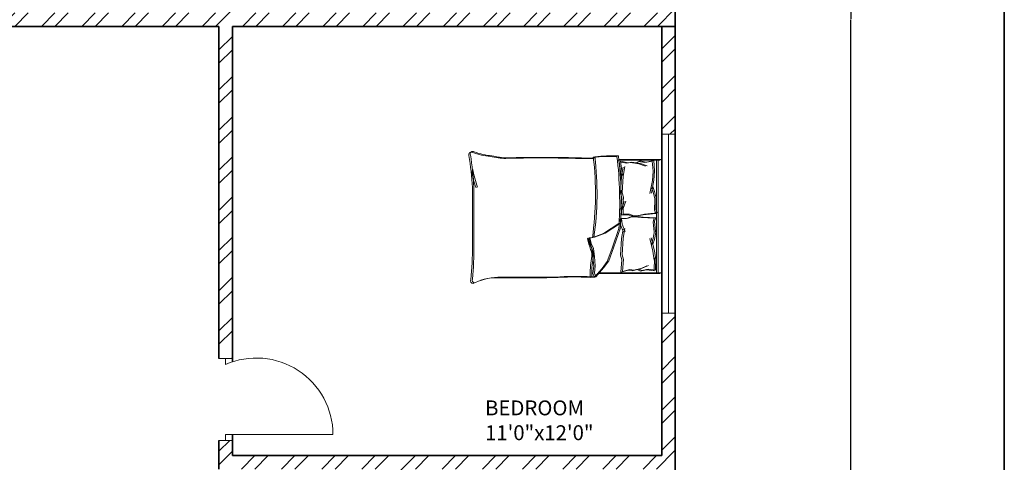
# Model space of a CAD drawing. Units: inches. Extents: x 1962 to 2771, y 1245 to 2660.
# Tile 61 of 114: x 2441 to 2771, y 1831 to 1979. Entities that reach past the tile are written whole.
import ezdxf

# ---------------------------------------------------------------- set-up
doc = ezdxf.new("R2010")
doc.units = ezdxf.units.IN
for name, color, linetype, lineweight in [('A-ANNO-DIMS', 2, 'Continuous', 18), ('A-ANNO-TTLB', 7, 'Continuous', 35), ('A-AREA-IDEN', 7, 'Continuous', 18), ('A-DOOR', 3, 'Continuous', 18), ('A-FURN', 8, 'Continuous', 13), ('A-GLAZ', 4, 'Continuous', 18), ('A-WALL', 7, 'Continuous', 35), ('A-WALL-PATT', 252, 'Continuous', 13)]:
    doc.layers.add(name, color=color, linetype=linetype, lineweight=lineweight)
doc.styles.get("Standard").update_dxf_attribs({"font": 'arial.ttf'})
doc.dimstyles.get("Standard").update_dxf_attribs({"dimtxt": 0.18, "dimasz": 0.18, "dimexe": 0.18, "dimexo": 0.0625, "dimgap": 0.09, "dimtad": 0, "dimtih": 1, "dimtoh": 1, "dimdec": 4, "dimzin": 0, "dimdsep": 46, "dimtxsty": 'Standard', "dimcen": 0.09, "dimadec": 0, "dimazin": 0, "dimtfac": 1, "dimtdec": 4, "dimtofl": 0, "dimtmove": 0, "dimatfit": 3, "dimfxl": 1, "dimtolj": 1, "dimtzin": 0, "dimarcsym": 0})

# ---------------------------------------------------------------- blocks, each defined once
blk = doc.blocks.new('BED-PLAN')
for p, q in [((0, 40.75), (21.15, 40.75)), ((0, 40.75), (21.15, 40.75)), ((0, 2.76), (0, 40.75)), ((0.51, 40.93), (21.66, 40.93)), ((0.51, 40.93), (21.66, 40.93)), ((1.22, 2.76), (1.22, 40.75)), ((1.22, 2.76), (1.22, 40.75)), ((1.73, 2.95), (1.73, 40.93)), ((1.73, 2.95), (1.73, 40.93)), ((2.03, 39.83), (1.96, 35.54)), ((2.03, 39.83), (1.96, 35.54)), ((2.03, 39.83), (4.58, 39.53)), ((2.03, 39.83), (4.58, 39.53)), ((2.54, 40.02), (2.46, 35.72)), ((2.54, 40.02), (2.46, 35.72)), ((2.54, 40.02), (5.09, 39.72)), ((2.54, 40.02), (5.09, 39.72)), ((4.58, 39.53), (6.63, 40.01)), ((4.58, 39.53), (6.63, 40.01)), ((5.09, 39.72), (7.14, 40.19)), ((5.09, 39.72), (7.14, 40.19)), ((9.4, 39.83), (6.56, 39.2)), ((9.4, 39.83), (6.56, 39.2)), ((6.63, 40.01), (7.46, 39.6)), ((6.63, 40.01), (7.46, 39.6)), ((9.91, 40.02), (7.07, 39.38)), ((9.91, 40.02), (7.07, 39.38)), ((7.14, 40.19), (7.97, 39.78)), ((7.14, 40.19), (7.97, 39.78)), ((10.68, 39.68), (9.4, 39.83)), ((10.68, 39.68), (9.4, 39.83)), ((11.19, 39.87), (9.91, 40.02)), ((11.19, 39.87), (9.91, 40.02)), ((13.17, 40.3), (10.68, 39.68)), ((13.17, 40.3), (10.68, 39.68)), ((13.68, 40.48), (11.19, 39.87)), ((13.68, 40.48), (11.19, 39.87)), ((12.85, 36.22), (13.17, 40.3)), ((12.85, 36.22), (13.17, 40.3)), ((13.36, 36.4), (13.68, 40.48)), ((13.36, 36.4), (13.68, 40.48)), ((22.05, 42.03), (19.47, 39.08)), ((22.05, 42.02), (19.47, 39.08)), ((22.56, 42.21), (19.98, 39.26)), ((22.56, 42.21), (19.98, 39.26)), ((23.44, 42.09), (22.05, 42.03, 3.08)), ((23.44, 42.09), (22.05, 42.02, 3.08)), ((22.55, 40.8), (22.05, 42.03)), ((22.55, 40.8), (22.05, 42.02)), ((22.3, 38.34), (22.55, 40.8)), ((22.3, 38.34), (22.55, 40.8)), ((23.95, 42.27), (22.56, 42.21, 3.08)), ((23.95, 42.27), (22.56, 42.21, 3.08)), ((23.06, 40.98), (22.56, 42.21)), ((23.06, 40.98), (22.56, 42.21)), ((22.81, 38.52), (23.06, 40.98)), ((22.81, 38.52), (23.06, 40.98)), ((1.96, 35.54), (2.02, 36.34)), ((1.96, 35.54), (2.02, 36.34)), ((2.02, 36.34), (2.44, 33.32)), ((2.02, 36.34), (2.44, 33.32)), ((2.46, 35.72), (2.53, 36.52)), ((2.46, 35.72), (2.53, 36.52)), ((2.53, 36.52), (2.95, 33.5)), ((2.53, 36.52), (2.95, 33.5)), ((6.56, 39.2), (4.43, 38.26)), ((6.56, 39.2), (4.43, 38.26)), ((7.07, 39.38), (4.94, 38.44)), ((7.07, 39.38), (4.94, 38.44)), ((13.8, 34.84), (13.36, 36.4)), ((13.8, 34.84), (13.36, 36.4)), ((17.75, 36.74), (16.15, 32.31)), ((17.75, 36.74), (16.15, 32.31)), ((18.26, 36.92), (16.66, 32.49)), ((18.26, 36.92), (16.66, 32.49)), ((19.47, 39.08), (17.75, 36.74)), ((19.47, 39.08), (17.75, 36.74)), ((19.98, 39.26), (18.26, 36.92)), ((19.98, 39.26), (18.26, 36.92)), ((22.55, 35.26), (22.3, 38.34)), ((22.55, 35.26), (22.3, 38.34)), ((23.06, 35.45), (22.81, 38.52)), ((23.06, 35.44), (22.81, 38.52)), ((2.44, 33.32), (3.52, 29.01)), ((2.44, 33.32), (3.52, 29.01)), ((2.95, 33.5), (4.02, 29.19)), ((2.95, 33.5), (4.02, 29.19)), ((13.3, 34.66), (12.85, 36.22)), ((13.3, 34.66), (12.85, 36.22)), ((12.95, 29.09), (13.3, 34.66)), ((12.95, 29.09), (13.3, 34.66)), ((13.46, 29.27), (13.8, 34.84)), ((13.46, 29.27), (13.8, 34.84)), ((22.92, 32.56), (22.55, 35.26)), ((22.92, 32.55), (22.55, 35.26)), ((23.42, 32.74), (23.06, 35.45)), ((23.42, 32.74), (23.06, 35.44)), ((2.92, 31.16), (2.45, 29.52)), ((2.92, 31.16), (2.45, 29.52)), ((3.43, 31.34), (2.96, 29.7)), ((3.43, 31.34), (2.96, 29.7)), ((16.15, 32.31), (13.82, 25.68)), ((16.15, 32.31), (13.82, 25.68)), ((16.66, 32.49), (14.33, 25.86)), ((16.66, 32.49), (14.33, 25.86)), ((23.65, 30.95), (22.92, 32.56)), ((23.65, 30.95), (22.92, 32.55)), ((24.16, 31.14), (23.42, 32.74)), ((24.16, 31.14), (23.42, 32.74)), ((24.15, 28.99), (23.65, 30.95)), ((24.15, 28.98), (23.65, 30.95)), ((24.65, 29.17), (24.16, 31.14)), ((24.65, 29.17), (24.16, 31.14)), ((62.99, 11.98), (62.99, 31.54)), ((62.99, 11.97), (62.99, 31.54)), ((63.5, 12.16), (63.5, 31.72)), ((63.5, 12.16), (63.5, 31.72)), ((2.45, 29.52), (2.02, 27.19)), ((2.45, 29.52), (2.02, 27.19)), ((2.02, 27.19), (2.03, 26.94)), ((2.02, 27.19), (2.03, 26.93)), ((2.03, 26.94), (2.37, 23.42)), ((2.03, 26.93), (2.37, 23.42)), ((2.96, 29.7), (2.52, 27.37)), ((2.96, 29.7), (2.52, 27.37)), ((2.52, 27.37), (2.54, 27.12)), ((2.52, 27.37), (2.54, 27.12)), ((2.54, 27.12), (2.88, 23.6)), ((2.54, 27.12), (2.88, 23.6)), ((13.31, 24.44), (12.28, 26.89)), ((13.31, 24.44), (12.28, 26.88)), ((12.42, 25.89), (12.95, 29.09)), ((12.42, 25.89), (12.95, 29.09)), ((13.81, 24.63), (12.79, 27.07)), ((13.81, 24.63), (12.79, 27.07)), ((12.93, 26.07), (13.46, 29.27)), ((12.93, 26.07), (13.46, 29.27)), ((13.82, 24.05), (18.98, 27.38)), ((13.82, 24.05), (18.98, 27.38)), ((14.33, 24.24), (19.49, 27.57)), ((14.33, 24.24), (19.49, 27.57)), ((18.98, 27.38), (22.55, 28.74)), ((18.98, 27.38), (22.55, 28.74)), ((19.49, 27.57), (23.06, 28.92)), ((19.49, 27.57), (23.06, 28.92)), ((22.55, 28.74), (24.15, 28.99)), ((22.55, 28.74), (24.15, 28.98)), ((23.06, 28.92), (24.65, 29.17)), ((23.06, 28.92), (24.65, 29.17)), ((2.37, 23.42), (1.98, 22.24)), ((2.37, 23.42), (1.98, 22.24)), ((2.88, 23.6), (2.49, 22.42)), ((2.88, 23.6), (2.49, 22.42)), ((13.43, 22.49), (13.31, 24.44)), ((13.43, 22.49), (13.31, 24.44)), ((13.94, 22.68), (13.81, 24.63)), ((13.94, 22.68), (13.81, 24.63)), ((1.49, 20.65), (5.74, 21.11)), ((1.49, 20.65), (5.74, 21.11)), ((1.95, 19.51), (1.49, 20.65)), ((1.95, 19.51), (1.49, 20.65)), ((1.98, 22.24), (6.25, 22.05)), ((1.98, 22.24), (6.25, 22.05)), ((1.99, 20.84), (6.25, 21.3)), ((1.99, 20.84), (6.25, 21.3)), ((2.45, 19.69), (1.99, 20.84)), ((2.45, 19.69), (1.99, 20.84)), ((2.49, 22.42), (6.76, 22.23)), ((2.49, 22.42), (6.76, 22.23)), ((5.74, 21.11), (8.27, 21.57)), ((5.74, 21.11), (8.27, 21.57)), ((6.25, 22.05), (8.81, 21.75)), ((6.25, 22.05), (8.81, 21.75)), ((6.25, 21.3), (8.78, 21.76)), ((6.25, 21.3), (8.78, 21.76)), ((6.76, 22.23), (9.31, 21.93)), ((6.76, 22.23), (9.31, 21.93)), ((8.27, 21.57), (9.3, 21.57)), ((8.27, 21.57), (9.3, 21.57)), ((8.78, 21.76), (9.81, 21.76)), ((8.78, 21.76), (9.81, 21.76)), ((8.81, 21.75), (9.84, 21.81)), ((8.81, 21.75), (9.84, 21.81)), ((9.3, 21.57), (10.8, 21.11)), ((9.3, 21.57), (10.8, 21.11)), ((9.31, 21.93), (10.35, 21.99)), ((9.31, 21.93), (10.35, 21.99)), ((9.81, 21.76), (11.3, 21.3)), ((9.81, 21.76), (11.3, 21.3)), ((9.84, 21.81), (11.3, 22.36)), ((9.84, 21.81), (11.3, 22.36)), ((10.35, 21.99), (11.81, 22.54)), ((10.35, 21.99), (11.81, 22.54)), ((10.8, 21.11), (12.93, 21.11)), ((10.8, 21.11), (12.93, 21.11)), ((11.3, 22.36), (13.43, 22.49)), ((11.3, 22.36), (13.43, 22.49)), ((11.3, 21.3), (13.44, 21.3)), ((11.3, 21.3), (13.44, 21.3)), ((11.81, 22.54), (13.94, 22.68)), ((11.81, 22.54), (13.94, 22.68)), ((12.93, 21.11), (12.93, 19.16)), ((12.93, 21.11), (12.93, 19.16)), ((13.44, 21.3), (13.44, 19.34)), ((13.44, 21.3), (13.44, 19.34)), ((1.83, 15.97), (1.95, 19.51)), ((1.83, 15.97), (1.95, 19.51)), ((2.34, 16.15), (2.45, 19.69)), ((2.34, 16.15), (2.45, 19.69)), ((12.93, 19.16), (12.06, 16.66)), ((12.93, 19.16), (12.06, 16.66)), ((13.44, 19.34), (12.57, 16.84)), ((13.44, 19.34), (12.57, 16.84)), ((12.85, 15.41), (13.17, 19.49)), ((12.85, 15.41), (13.17, 19.49)), ((13.36, 15.59), (13.68, 19.67)), ((13.36, 15.59), (13.68, 19.67)), ((1.83, 15.72), (1.83, 15.97)), ((1.83, 15.72), (1.83, 15.97)), ((2.41, 13.42), (1.83, 15.72)), ((2.41, 13.42), (1.83, 15.72)), ((2.34, 15.9), (2.34, 16.15)), ((2.34, 15.9), (2.34, 16.15)), ((2.91, 13.6), (2.34, 15.9)), ((2.91, 13.6), (2.34, 15.9)), ((2.98, 11.81), (2.41, 13.42)), ((2.98, 11.81), (2.41, 13.42)), ((2.64, 9.63), (3.44, 13.99)), ((2.64, 9.63), (3.44, 13.99)), ((3.49, 11.99), (2.91, 13.6)), ((3.49, 11.99), (2.91, 13.6)), ((3.14, 9.81), (3.95, 14.17)), ((3.14, 9.81), (3.95, 14.17)), ((13.3, 13.85), (12.85, 15.41)), ((13.3, 13.85), (12.85, 15.41)), ((12.95, 8.28), (13.3, 13.85)), ((12.95, 8.28), (13.3, 13.85)), ((13.8, 14.03), (13.36, 15.59)), ((13.8, 14.03), (13.36, 15.59)), ((13.46, 8.46), (13.8, 14.03)), ((13.46, 8.46), (13.8, 14.03)), ((2.41, 6.59), (2.64, 9.63)), ((2.41, 6.59), (2.64, 9.63)), ((2.9, 6.68), (2.91, 6.77)), ((2.9, 6.68), (2.91, 6.77)), ((3.16, 3.28), (2.9, 6.68)), ((3.16, 3.28), (2.9, 6.68)), ((2.91, 6.77), (3.14, 9.81)), ((2.91, 6.77), (3.14, 9.81)), ((12.42, 5.07), (12.95, 8.28)), ((12.42, 5.07), (12.95, 8.28)), ((12.93, 5.26), (13.46, 8.46)), ((12.93, 5.26), (13.46, 8.46)), ((12.95, 8.28), (13.21, 7.38)), ((12.95, 8.28), (13.21, 7.38)), ((13.21, 7.38), (13.78, 3.33)), ((13.21, 7.38), (13.78, 3.33)), ((13.46, 8.46), (13.72, 7.56)), ((13.46, 8.46), (13.72, 7.56)), ((13.72, 7.56), (14.29, 3.51)), ((13.72, 7.56), (14.29, 3.51)), ((2.39, 6.5), (2.41, 6.59)), ((2.39, 6.5), (2.41, 6.59)), ((2.65, 3.1), (2.39, 6.5)), ((2.65, 3.1), (2.39, 6.5)), ((2.64, 3.1), (5.16, 3.56)), ((2.64, 3.1), (5.16, 3.56)), ((3.14, 3.28), (5.67, 3.74)), ((3.14, 3.28), (5.67, 3.74)), ((7.12, 4.02), (4.93, 4.82)), ((7.12, 4.02), (4.93, 4.82)), ((5.16, 3.56), (7.23, 3.21)), ((5.16, 3.56), (7.23, 3.21)), ((7.63, 4.2), (5.44, 5)), ((7.63, 4.2), (5.44, 5)), ((5.67, 3.74), (7.74, 3.39)), ((5.67, 3.74), (7.74, 3.39)), ((9.99, 3.56), (7.12, 4.02)), ((9.99, 3.56), (7.12, 4.02)), ((7.23, 3.21), (8.04, 3.67)), ((7.23, 3.21), (8.04, 3.67)), ((10.5, 3.74), (7.63, 4.2)), ((10.5, 3.74), (7.63, 4.2)), ((7.74, 3.39), (8.55, 3.85)), ((7.74, 3.39), (8.55, 3.85)), ((11.26, 3.79), (9.99, 3.56)), ((11.26, 3.79), (9.99, 3.56)), ((11.76, 3.97), (10.5, 3.74)), ((11.76, 3.97), (10.5, 3.74)), ((13.78, 3.33), (11.26, 3.79)), ((13.78, 3.33), (11.26, 3.79)), ((14.29, 3.51), (11.76, 3.97)), ((14.29, 3.51), (11.76, 3.97)), ((14.4, 2.76), (0, 2.76)), ((14.4, 2.76), (0, 2.76)), ((14.9, 2.95), (0.51, 2.95)), ((14.9, 2.95), (0.51, 2.95))]:
    blk.add_line(p, q)
for centre, radius, start, end in [((54.58, 60.54), 18.33, 267.4714, 296.4681), ((54.58, 60.54), 18.33, 267.4714, 296.4681), ((55.09, 60.72), 18.33, 267.4714, 296.4681), ((55.09, 60.72), 18.33, 267.4714, 296.4681), ((62.69, 43.25), 0.876, 332.6588, 86.02), ((62.69, 43.25), 0.876, 332.6588, 86.02), ((63.2, 43.43), 0.876, 332.6588, 86.02), ((63.2, 43.43), 0.876, 332.6588, 86.02), ((169.24, 32.89), 105.75, 174.4998, 180.6351), ((169.24, 32.89), 105.75, 174.4998, 180.6351), ((-5.29, 40.8), 28.76, 349.8763, 2.5657), ((-5.29, 40.8), 28.76, 349.8763, 2.5657), ((28.87, 144.88), 102.94, 266.9791, 273.8365), ((28.87, 144.88), 102.94, 266.9791, 273.8365), ((-4.78, 40.98), 28.76, 349.8763, 2.5657), ((-4.78, 40.98), 28.76, 349.8763, 2.5657), ((29.37, 145.06), 102.94, 266.9791, 273.8365), ((29.37, 145.06), 102.94, 266.9791, 273.8365), ((53.91, -3583.94), 3626.16, 90.00217, 90.28689), ((53.91, -3583.94), 3626.16, 90.00217, 90.28689), ((54.42, -3583.75), 3626.16, 90.00217, 90.28689), ((54.42, -3583.75), 3626.16, 90.00217, 90.28689), ((168.74, 32.71), 105.75, 174.4998, 180.6351), ((168.74, 32.71), 105.75, 174.4998, 180.6351), ((27.87, 34.77), 4.95, 168.6608, 203.7384), ((27.87, 34.77), 4.95, 168.6608, 203.7384), ((28.38, 34.95), 4.95, 168.6608, 203.7384), ((28.38, 34.95), 4.95, 168.6608, 203.7384), ((1.18, 24.77), 23.57, 10.6617, 19.8806), ((1.18, 24.76), 23.57, 10.6617, 19.8806), ((1.69, 24.95), 23.57, 10.6617, 19.8806), ((1.69, 24.95), 23.57, 10.6617, 19.8806), ((124.25, 14.12), 102.56, 171.7845, 186.9006), ((124.25, 14.11), 102.56, 171.7845, 186.9006), ((124.76, 14.3), 102.56, 171.7845, 186.9006), ((124.76, 14.3), 102.56, 171.7845, 186.9006), ((24.2, 29.12), 0.147, 250.2464, 1.1377), ((24.2, 29.12), 0.147, 250.2464, 1.1377), ((24.7, 29.3), 0.147, 250.2464, 1.1377), ((24.7, 29.3), 0.147, 250.2464, 1.1377), ((144.71, 16.98), 131.13, 176.0865, 186.7821), ((144.71, 16.98), 131.13, 176.0865, 186.7821), ((145.22, 17.16), 131.13, 176.0865, 186.7821), ((145.22, 17.16), 131.13, 176.0865, 186.7821), ((-18.85, -13.69), 84.62, 13.3832, 17.7053), ((-18.85, -13.69), 84.62, 13.3832, 17.7053), ((-18.34, -13.51), 84.62, 13.3832, 17.7053), ((-18.34, -13.51), 84.62, 13.3832, 17.7053), ((159.64, 17.03), 96.78, 182.9958, 189.4091), ((159.64, 17.03), 96.78, 182.9958, 189.4091), ((160.15, 17.21), 96.78, 182.9958, 189.4091), ((160.15, 17.21), 96.78, 182.9958, 189.4091), ((15.97, 67.7), 66.22, 268.7218, 275.604), ((15.97, 67.7), 66.22, 268.7218, 275.604), ((16.48, 67.88), 66.22, 268.7218, 275.604), ((16.48, 67.88), 66.22, 268.7218, 275.604), ((24.78, -132.99), 135.22, 88.4762, 91.0082), ((24.78, -132.99), 135.22, 88.4762, 91.0082), ((25.29, -132.81), 135.22, 88.4762, 91.0082), ((25.29, -132.81), 135.22, 88.4762, 91.0082), ((40.23, 385.38), 383.38, 268.2277, 271.7185), ((40.23, 385.38), 383.38, 268.2277, 271.7185), ((40.74, 385.56), 383.38, 268.2277, 271.7185), ((40.74, 385.56), 383.38, 268.2277, 271.7185), ((51.28, -21.38), 23.56, 76.0648, 88.9113), ((51.28, -21.38), 23.56, 76.0648, 88.9113), ((51.79, -21.2), 23.56, 76.0648, 88.9113), ((51.79, -21.2), 23.56, 76.0648, 88.9113), ((55.86, -17.22), 18.73, 67.9751, 86.652), ((55.86, -17.22), 18.73, 67.9751, 86.652), ((56.37, -17.03), 18.73, 67.9751, 86.652), ((56.37, -17.03), 18.73, 67.9751, 86.652), ((63.37, 0.87), 0.866, 236.1736, 23.4781), ((63.37, 0.87), 0.866, 236.1736, 23.4781), ((63.87, 1.05), 0.866, 236.1736, 23.4781), ((63.87, 1.05), 0.866, 236.1736, 23.4781)]:
    blk.add_arc(centre, radius, start, end)
blk = doc.blocks.new('WIN-60IN-A')
for p, q in [((0, 60), (4.5, 60)), ((4.5, 60), (2.25, 60)), ((2.25, 60), (2.25, 0)), ((2.25, 0), (0, 0)), ((0, 0), (4.5, 0))]:
    blk.add_line(p, q)
blk = doc.blocks.new('*D42')
at = {"layer": 'A-ANNO-DIMS', "color": 0, "lineweight": -2, "transparency": 16777216}
for p, q in [((2660.87, 2524.34), (2719.94, 2524.34)), ((2719.76, 2524.16), (2719.76, 1979.28)), ((2719.76, 1434.02), (2719.76, 1978.91)), ((2660.87, 1433.84), (2719.94, 1433.84))]:
    blk.add_line(p, q, dxfattribs=at)
at = {"layer": 'A-ANNO-DIMS', "color": 0, "transparency": 16777216}
for points in [[(2719.73, 2524.16), (2719.79, 2524.16), (2719.76, 2524.34)], [(2719.73, 1434.02), (2719.79, 1434.02), (2719.76, 1433.84)]]:
    blk.add_solid(points, dxfattribs=at)
at = {"layer": 'Defpoints', "color": 0, "transparency": 16777216}
for p in [(2660.81, 2524.34), (2719.76, 2524.34), (2660.81, 1433.84)]:
    blk.add_point(p, dxfattribs=at)
at = {"layer": 'A-ANNO-DIMS', "color": 0, "transparency": 16777216, "insert": (2719.76, 1979.09), "char_height": 0.18, "attachment_point": 5}
blk.add_mtext('\\A1;1090.5', dxfattribs=at)

msp = doc.modelspace()

# ---------------------------------------------------------------- hatches: boundary and pattern name
at = {"layer": 'A-WALL-PATT'}
h = msp.add_hatch(dxfattribs=at)
h.set_pattern_fill('ANSI32', color=256)
h.paths.add_polyline_path([(2090.8074, 2467.3437), (2141.6481, 2467.3437), (2141.6481, 2469.5937), (2141.6481, 2471.8437), (2086.3074, 2471.8437), (2086.3074, 2422.5333), (2090.8074, 2422.5333)])
h.paths.add_polyline_path([(2282.7664, 2471.8437), (2204.8982, 2471.8437), (2204.8982, 2467.3437), (2234.8074, 2467.3437), (2234.8074, 2311.3437), (2228.7492, 2311.3437), (2228.7492, 2306.8437), (2234.8074, 2306.8437), (2331.9227, 2306.8437), (2331.9227, 2309.0937), (2331.9227, 2311.3437), (2239.3074, 2311.3437), (2239.3074, 2467.3437), (2282.7664, 2467.3437), (2282.7664, 2469.5937)])
h.paths.add_polyline_path([(2471.4531, 2519.8437), (2552.011, 2519.8437), (2564.3996, 2519.8437), (2564.3996, 2511.1389), (2568.8996, 2511.1389), (2568.8996, 2524.3437), (2466.9531, 2524.3437), (2466.9531, 2471.8437), (2450.0749, 2471.8437), (2446.4672, 2471.8437), (2446.4672, 2467.3437), (2450.0749, 2467.3437), (2475.9988, 2467.3437), (2475.9988, 2469.5937), (2475.9988, 2471.8437), (2471.4531, 2471.8437)])
h.paths.add_polyline_path([(2575.2231, 2469.5937), (2575.2231, 2471.8437), (2568.8996, 2471.8437), (2568.8996, 2487.1389), (2564.3996, 2487.1389), (2564.3996, 2471.8437), (2556.511, 2471.8437), (2499.2904, 2471.8437), (2499.2904, 2467.3437), (2507.8074, 2467.3437), (2507.8074, 2311.3437), (2414.863, 2311.3437), (2414.863, 2306.8437), (2512.3074, 2306.8437), (2517.0114, 2306.8437), (2517.0114, 2309.0937), (2517.0114, 2311.3437), (2512.3074, 2311.3437), (2512.3074, 2467.3437), (2575.2231, 2467.3437)])
h.paths.add_polyline_path([(2660.8074, 2471.8437), (2600.9602, 2471.8437), (2600.9602, 2467.3437), (2656.3074, 2467.3437), (2656.3074, 2432.5704), (2660.8074, 2432.5704)])
h.paths.add_polyline_path([(2660.8074, 2372.5704), (2656.3074, 2372.5704), (2656.3074, 2311.3437), (2600.276, 2311.3437), (2600.276, 2309.0937), (2600.276, 2306.8437), (2656.3074, 2306.8437), (2656.3074, 2296.2593), (2660.8074, 2296.2593)])
h.paths.add_polyline_path([(2572.3074, 2306.8437), (2577.1385, 2306.8437), (2577.1385, 2311.3437), (2551.082, 2311.3437), (2551.082, 2306.8437), (2567.8074, 2306.8437), (2567.8074, 2258.8437), (2540.0574, 2258.8437), (2540.0574, 2256.5937), (2540.0574, 2254.3437), (2567.8074, 2254.3437), (2656.3074, 2254.3437), (2656.3074, 2236.9085), (2660.8074, 2236.9085), (2660.8074, 2272.2593), (2656.3074, 2272.2593), (2656.3074, 2258.8437), (2572.3074, 2258.8437)])
h.paths.add_polyline_path([(2512.3074, 2254.3437), (2518.8716, 2254.3437), (2518.8716, 2256.5937), (2518.8716, 2258.8437), (2507.8074, 2258.8437), (2507.8074, 2177.8437), (2567.8074, 2177.8437), (2567.8074, 2172.9628), (2572.3074, 2172.9628), (2572.3074, 2177.8437), (2656.3074, 2177.8437), (2656.3074, 2166.4846), (2660.8074, 2166.4846), (2660.8074, 2200.9085), (2656.3074, 2200.9085), (2656.3074, 2182.3437), (2512.3074, 2182.3437)])
h.paths.add_polyline_path([(2656.3074, 2129.8437), (2572.3074, 2129.8437), (2572.3074, 2150.3044), (2570.0574, 2150.3044), (2567.8074, 2150.3044), (2567.8074, 2129.8437), (2507.8074, 2129.8437), (2507.8074, 2116.3027), (2510.0574, 2116.3027), (2512.3074, 2116.3027), (2512.3074, 2125.3437), (2567.8074, 2125.3437), (2572.3074, 2125.3437), (2656.3074, 2125.3437)])
h.paths.add_polyline_path([(2090.8074, 2362.5333), (2086.3074, 2362.5333), (2086.3074, 2298.6242), (2090.8074, 2298.6242), (2090.8074, 2306.8437), (2174.8074, 2306.8437), (2174.8074, 2286.4178), (2179.3074, 2286.4178), (2179.3074, 2306.8437), (2192.8641, 2306.8437), (2192.8641, 2309.0937), (2192.8641, 2311.3437), (2090.8074, 2311.3437)])
h.paths.add_polyline_path([(2209.156, 2258.8437), (2179.3074, 2258.8437), (2179.3074, 2263.2236), (2177.0574, 2263.2236), (2174.8074, 2263.2236), (2174.8074, 2258.8437), (2090.8074, 2258.8437), (2090.8074, 2274.6242), (2086.3074, 2274.6242), (2086.3074, 2238.2967), (2088.5574, 2238.2967), (2090.8074, 2238.2967), (2090.8074, 2254.3437), (2209.156, 2254.3437)])
h.paths.add_polyline_path([(2090.8074, 2177.8437), (2234.8074, 2177.8437), (2234.8074, 2173.1428), (2239.3074, 2173.1428), (2239.3074, 2258.8437), (2230.8442, 2258.8437), (2230.8442, 2256.5937), (2230.8442, 2254.3437), (2234.8074, 2254.3437), (2234.8074, 2182.3437), (2090.8074, 2182.3437), (2090.8074, 2202.2967), (2086.3074, 2202.2967), (2086.3074, 2140.0389), (2090.8074, 2140.0389)])
h.paths.add_polyline_path([(2090.8074, 2080.0389), (2086.3074, 2080.0389), (2086.3074, 2033.8437), (2090.8074, 2033.8437)], flags=17)
h.paths.add_polyline_path([(2244.9405, 2033.8437), (2239.3074, 2033.8437), (2239.3074, 2142.0665), (2237.2592, 2142.0665), (2234.8074, 2142.0665), (2234.8074, 2033.8437), (2090.8074, 2033.8437), (2076.5204, 2033.8437), (2072.0204, 2033.8437), (2072.0204, 2000.4493), (2076.5204, 2000.4493), (2076.5204, 2029.3437), (2090.8074, 2029.3437), (2244.9405, 2029.3437), (2244.9405, 2031.5937)])
h.paths.add_polyline_path([(2234.8074, 1933.3437), (2076.5204, 1933.3437), (2076.5204, 1952.4493), (2074.2704, 1952.4493), (2072.0204, 1952.4493), (2072.0204, 1933.3437), (2072.0204, 1928.8437), (2234.8074, 1928.8437)])
h.paths.add_polyline_path([(2090.8074, 1928.8437), (2086.3074, 1928.8437), (2086.3074, 1906.5013), (2090.8074, 1906.5013)])
h.paths.add_polyline_path([(2090.8074, 1846.5013), (2086.3074, 1846.5013), (2086.3074, 1769.9917), (2088.5574, 1769.9917), (2090.8074, 1769.9917), (2090.8074, 1780.3437), (2234.8074, 1780.3437), (2234.8074, 1708.3437), (2230.3764, 1708.3437), (2230.3764, 1703.8437), (2239.3074, 1703.8437), (2239.3074, 1792.6669), (2237.0574, 1792.6669), (2234.8074, 1792.6669), (2234.8074, 1784.8437), (2090.8074, 1784.8437)])
h.paths.add_polyline_path([(2239.3074, 1928.8437), (2244.9405, 1928.8437), (2244.9405, 1931.0937), (2244.9405, 1933.3437), (2234.8074, 1933.3437), (2234.8074, 1928.8437), (2234.8074, 1825.5949), (2239.3074, 1825.5949)])
h.paths.add_polyline_path([(2148.0425, 1649.0937), (2148.0425, 1651.3437), (2090.8074, 1651.3437), (2090.8074, 1646.8437), (2148.0425, 1646.8437)], flags=0)
h.paths.add_polyline_path([(2207.5601, 1708.3437), (2090.8074, 1708.3437), (2090.8074, 1703.8437), (2174.8074, 1703.8437), (2174.8074, 1651.3437), (2170.4457, 1651.3437), (2170.4457, 1646.8437), (2195.9924, 1646.8437), (2195.9924, 1649.0937), (2195.9924, 1651.3437), (2179.3074, 1651.3437), (2179.3074, 1703.8437), (2207.5601, 1703.8437), (2207.5601, 1706.0937)])
h.paths.add_polyline_path([(2090.8074, 1733.9917), (2086.3074, 1733.9917), (2086.3074, 1696.1032), (2088.5574, 1696.1032), (2090.8074, 1696.1032)])
h.paths.add_polyline_path([(2090.8074, 1672.1032), (2086.3074, 1672.1032), (2086.3074, 1600.3335), (2090.8074, 1600.3335)])
h.paths.add_polyline_path([(2090.8074, 1540.3335), (2086.3074, 1540.3335), (2086.3074, 1486.3437), (2139.6766, 1486.3437), (2139.6766, 1490.8437), (2090.8074, 1490.8437)])
h.paths.add_polyline_path([(2302.3876, 1490.8437), (2239.3074, 1490.8437), (2239.3074, 1646.8437), (2335.9994, 1646.8437), (2335.9994, 1651.3437), (2229.884, 1651.3437), (2229.884, 1646.8437), (2234.8074, 1646.8437), (2234.8074, 1490.8437), (2202.7103, 1490.8437), (2202.7103, 1488.5937), (2202.7103, 1486.3437), (2275.0699, 1486.3437), (2275.0699, 1475.772), (2279.5699, 1475.772), (2279.5699, 1486.3437), (2302.3876, 1486.3437)])
h.paths.add_polyline_path([(2279.5699, 1451.772), (2275.0699, 1451.772), (2275.0699, 1438.3437), (2174.8074, 1438.3437), (2174.8074, 1486.3437), (2179.7922, 1486.3437), (2179.7922, 1490.8437), (2163.3585, 1490.8437), (2163.3585, 1488.5937), (2163.3585, 1486.3437), (2170.3074, 1486.3437), (2170.3074, 1433.8437), (2279.5699, 1433.8437)])
h.paths.add_polyline_path([(2427.2363, 1490.8437), (2375.8074, 1490.8437), (2375.8074, 1646.8437), (2381.6401, 1646.8437), (2381.6401, 1651.3437), (2365.887, 1651.3437), (2365.887, 1649.0937), (2365.887, 1646.8437), (2371.3074, 1646.8437), (2371.3074, 1490.8437), (2327.5627, 1490.8437), (2327.5627, 1488.5937), (2327.5627, 1486.3437), (2371.3074, 1486.3437), (2371.3074, 1433.8437), (2375.8074, 1433.8437), (2375.8074, 1486.3437), (2427.2363, 1486.3437)])
h.paths.add_polyline_path([(2512.3074, 1646.8437), (2519.4351, 1646.8437), (2519.4351, 1649.0937), (2519.4351, 1651.3437), (2507.8074, 1651.3437), (2416.0063, 1651.3437), (2416.0063, 1649.0937), (2416.0063, 1646.8437), (2507.8074, 1646.8437), (2507.8074, 1490.8437), (2497.0532, 1490.8437), (2497.0532, 1488.5937), (2497.0532, 1486.3437), (2574.9344, 1486.3437), (2574.9344, 1476.0181), (2579.4344, 1476.0181), (2579.4344, 1486.3437), (2584.4872, 1486.3437), (2584.3074, 1490.8437), (2512.3074, 1490.8437)])
h.paths.add_polyline_path([(2470.5091, 1486.3437), (2473.9767, 1486.3437), (2473.9767, 1490.8437), (2449.6605, 1490.8437), (2449.6605, 1488.5937), (2449.6605, 1486.3437), (2466.0091, 1486.3437), (2466.0091, 1433.8437), (2470.5091, 1433.8437), (2579.4344, 1433.8437), (2579.4344, 1452.0181), (2574.9344, 1452.0181), (2574.9344, 1438.3437), (2554.5091, 1438.3437), (2470.5091, 1438.3437)])
h.paths.add_polyline_path([(2656.3074, 1490.8437), (2611.86, 1490.8437), (2611.86, 1486.3437), (2656.3074, 1486.3437)])
h.paths.add_polyline_path([(2660.8074, 1532.7007), (2658.5574, 1532.7007), (2656.3074, 1532.7007), (2656.3074, 1486.3437), (2660.8074, 1486.3437)])
h.paths.add_polyline_path([(2660.8074, 1664.9663), (2656.3074, 1664.9663), (2656.3074, 1651.3437), (2602.2313, 1651.3437), (2602.2313, 1646.8437), (2656.3074, 1646.8437), (2656.3074, 1592.7007), (2660.8074, 1592.7007)])
h.paths.add_polyline_path([(2660.8074, 1724.5221), (2656.3074, 1724.5221), (2656.3074, 1703.8437), (2542.4725, 1703.8437), (2542.4725, 1699.3437), (2567.8074, 1699.3437), (2567.8074, 1651.3437), (2552.7766, 1651.3437), (2552.7766, 1649.0937), (2552.7766, 1646.8437), (2577.2878, 1646.8437), (2577.2878, 1649.0937), (2577.2878, 1651.3437), (2572.3074, 1651.3437), (2572.3074, 1699.3437), (2656.3074, 1699.3437), (2656.3074, 1688.9663), (2660.8074, 1688.9663)])
h.paths.add_polyline_path([(2660.8074, 1880.6524), (2656.3074, 1880.6524), (2656.3074, 1832.8437), (2512.3074, 1832.8437), (2512.3074, 1837.8959), (2507.8074, 1837.8959), (2507.8074, 1828.3437), (2567.8074, 1828.3437), (2567.8074, 1804.3437), (2572.3074, 1804.3437), (2572.3074, 1828.3437), (2656.3074, 1828.3437), (2656.3074, 1818.6778), (2660.8074, 1818.6778)])
h.paths.add_polyline_path([(2660.8074, 1794.6778), (2656.3074, 1794.6778), (2656.3074, 1780.3437), (2572.3074, 1780.3437), (2572.3074, 1783.0303), (2570.0574, 1783.0303), (2567.8074, 1783.0303), (2567.8074, 1780.3437), (2507.8074, 1780.3437), (2507.8074, 1699.3437), (2517.8858, 1699.3437), (2517.8858, 1701.5937), (2517.8858, 1703.8437), (2512.3074, 1703.8437), (2512.3074, 1775.8437), (2656.3074, 1775.8437), (2656.3074, 1760.5221), (2660.8074, 1760.5221)])
h.paths.add_polyline_path([(2660.8074, 1981.3437), (2660.8074, 2020.2808), (2658.5574, 2020.2808), (2656.3074, 2020.2808), (2656.3074, 1981.3437), (2512.3074, 1981.3437), (2512.3074, 2086.6996), (2507.8074, 2086.6996), (2507.8074, 1981.3437), (2375.8074, 1981.3437), (2375.8074, 1986.8505), (2373.5574, 1986.8505), (2371.3074, 1986.8505), (2371.3074, 1973.2607), (2375.8074, 1973.2607), (2375.8074, 1976.8437), (2507.8074, 1976.8437), (2507.8074, 1865.4281), (2510.0574, 1865.4281), (2512.3074, 1865.4281), (2512.3074, 1976.8437), (2660.8074, 1976.8437)])
h.paths.add_polyline_path([(2375.8074, 1940.297), (2373.5574, 1940.297), (2371.3074, 1940.297), (2371.3074, 1933.3437), (2278.4434, 1933.3437), (2278.4434, 1928.8437), (2371.3074, 1928.8437), (2371.3074, 1651.3437), (2375.8074, 1651.3437)])
h.paths.add_polyline_path([(2660.8074, 1976.8437), (2656.3074, 1976.8437), (2656.3074, 1940.6524), (2660.8074, 1940.6524)], flags=17)
h.paths.add_polyline_path([(2660.8074, 2142.4846), (2656.3074, 2142.4846), (2656.3074, 2080.2808), (2660.8074, 2080.2808)])
h.paths.add_polyline_path([(2381.4189, 2311.3437), (2375.8074, 2311.3437), (2375.8074, 2467.3437), (2424.7242, 2467.3437), (2424.7242, 2469.5937), (2424.7242, 2471.8437), (2375.8074, 2471.8437), (2375.8074, 2524.3437), (2371.3074, 2524.3437), (2371.3074, 2471.8437), (2307.2097, 2471.8437), (2307.2097, 2467.3437), (2371.3074, 2467.3437), (2371.3074, 2311.3437), (2366.8901, 2311.3437), (2366.8901, 2306.8437), (2371.3074, 2306.8437), (2371.3074, 2033.8437), (2279.6589, 2033.8437), (2279.6589, 2029.3437), (2371.3074, 2029.3437), (2371.3074, 2014.2598), (2375.8074, 2014.2598), (2375.8074, 2306.8437), (2381.4189, 2306.8437)])
h.paths.add_polyline_path([(2263.3074, 2524.3437), (2170.3074, 2524.3437), (2170.3074, 2519.8437), (2170.3074, 2471.8437), (2165.0312, 2471.8437), (2165.0312, 2467.3437), (2179.6721, 2467.3437), (2179.6721, 2469.5161), (2179.6721, 2471.8437), (2174.8074, 2471.8437), (2174.8074, 2519.8437), (2258.8074, 2519.8437), (2258.8074, 2511.6436), (2263.3074, 2511.6436)])
h.paths.add_polyline_path([(2245.0232, 1361.4123), (2492.9468, 1361.4123), (2492.9468, 1398.505), (2245.0232, 1398.505)], flags=9)
h.paths.add_polyline_path([(2388.1434, 2086.6936), (2425.0704, 2086.6936), (2425.0704, 2105.3509), (2388.1434, 2105.3509)], flags=9)
h.paths.add_polyline_path([(2404.922, 2242.6744), (2445.7337, 2242.6744), (2445.7337, 2261.3318), (2404.922, 2261.3318)], flags=9)
h.paths.add_polyline_path([(2269.4107, 2156.7935), (2306.3378, 2156.7935), (2306.3378, 2175.4508), (2269.4107, 2175.4508)], flags=9)
h.paths.add_polyline_path([(2269.3277, 2233.4343), (2306.2547, 2233.4343), (2306.2547, 2252.0917), (2269.3277, 2252.0917)], flags=9)
h.paths.add_polyline_path([(2431.6052, 2320.6922), (2470.4456, 2320.6922), (2470.4456, 2339.3495), (2431.6052, 2339.3495)], flags=25)
h.paths.add_polyline_path([(2249.6902, 2315.7608), (2288.5306, 2315.7608), (2288.5306, 2334.4182), (2249.6902, 2334.4182)], flags=25)
h.paths.add_polyline_path([(2096.9301, 2314.3181), (2135.7704, 2314.3181), (2135.7704, 2332.9755), (2096.9301, 2332.9755)], flags=25)
h.paths.add_polyline_path([(2134.3475, 2285.7089), (2161.4655, 2285.7089), (2161.4655, 2304.3662), (2134.3475, 2304.3662)], flags=9)
h.paths.add_polyline_path([(2126.5155, 2209.4076), (2159.9227, 2209.4076), (2159.9227, 2228.065), (2126.5155, 2228.065)], flags=25)
h.paths.add_polyline_path([(2110.5753, 2141.5299), (2149.4157, 2141.5299), (2149.4157, 2160.1872), (2110.5753, 2160.1872)], flags=25)
h.paths.add_polyline_path([(2249.8618, 1968.3317), (2286.3966, 1968.3317), (2286.3966, 1986.989), (2249.8618, 1986.989)], flags=9)
h.paths.add_polyline_path([(2395.9507, 1777.0051), (2436.7624, 1777.0051), (2436.7624, 1795.6625), (2395.9507, 1795.6625)], flags=9)
h.paths.add_polyline_path([(2398.5259, 1888.5651), (2435.0062, 1888.5651), (2435.0062, 1907.2224), (2398.5259, 1907.2224)], flags=25)
h.paths.add_polyline_path([(2259.3506, 1728.3559), (2296.2776, 1728.3559), (2296.2776, 1747.0132), (2259.3506, 1747.0132)], flags=9)
h.paths.add_polyline_path([(2271.3698, 1845.268), (2308.2968, 1845.268), (2308.2968, 1863.9253), (2271.3698, 1863.9253)], flags=9)
h.paths.add_polyline_path([(2120.9355, 1786.3027), (2159.7759, 1786.3027), (2159.7759, 1804.9601), (2120.9355, 1804.9601)], flags=25)
h.paths.add_polyline_path([(2121.3164, 1732.1043), (2154.7236, 1732.1043), (2154.7236, 1750.7616), (2121.3164, 1750.7616)], flags=25)
h.paths.add_polyline_path([(2118.3706, 1678.8997), (2147.5282, 1678.8997), (2147.5282, 1697.557), (2118.3706, 1697.557)], flags=25)
h.paths.add_polyline_path([(2385.9227, 1493.557), (2424.763, 1493.557), (2424.763, 1512.2143), (2385.9227, 1512.2143)], flags=25)
h.paths.add_polyline_path([(2248.7058, 1500.0256), (2287.5462, 1500.0256), (2287.5462, 1518.6829), (2248.7058, 1518.6829)], flags=25)
h.paths.add_polyline_path([(2104.1669, 1617.3771), (2143.0073, 1617.3771), (2143.0073, 1636.0344), (2104.1669, 1636.0344)], flags=9)
h.paths.add_polyline_path([(2096.0714, 1447.8824), (2137.3845, 1447.8824), (2137.3845, 1458.1859), (2096.0714, 1458.1859)], flags=9)
h.paths.add_polyline_path([(2180.6114, 1440.325), (2209.7689, 1440.325), (2209.7689, 1458.9823), (2180.6114, 1458.9823)], flags=25)
h.paths.add_polyline_path([(2316.1698, 1447.9637), (2357.4829, 1447.9637), (2357.4829, 1458.2673), (2316.1698, 1458.2673)], flags=9)
h.paths.add_polyline_path([(2397.6187, 1447.9637), (2438.9318, 1447.9637), (2438.9318, 1458.2673), (2397.6187, 1458.2673)], flags=9)
h.paths.add_polyline_path([(2473.0778, 1439.5953), (2502.2354, 1439.5953), (2502.2354, 1458.2527), (2473.0778, 1458.2527)], flags=25)
h.paths.add_polyline_path([(2589.7027, 1447.8819), (2631.0158, 1447.8819), (2631.0158, 1458.1855), (2589.7027, 1458.1855)], flags=9)
h.paths.add_polyline_path([(2522.4009, 1497.5285), (2561.2413, 1497.5285), (2561.2413, 1516.1859), (2522.4009, 1516.1859)], flags=25)
h.paths.add_polyline_path([(2579.6565, 1671.3482), (2608.8141, 1671.3482), (2608.8141, 1690.0056), (2579.6565, 1690.0056)], flags=25)
h.paths.add_polyline_path([(2544.7038, 1725.5064), (2578.1111, 1725.5064), (2578.1111, 1744.1637), (2544.7038, 1744.1637)], flags=25)
h.paths.add_polyline_path([(2578.1191, 1807.472), (2607.2766, 1807.472), (2607.2766, 1826.1293), (2578.1191, 1826.1293)], flags=25)
h.paths.add_polyline_path([(2595.0614, 1835.1839), (2633.9018, 1835.1839), (2633.9018, 1853.8413), (2595.0614, 1853.8413)], flags=25)
h.paths.add_polyline_path([(2567.0097, 2097.7035), (2605.8501, 2097.7035), (2605.8501, 2116.3609), (2567.0097, 2116.3609)], flags=9)
h.paths.add_polyline_path([(2586.644, 2134.6454), (2615.8015, 2134.6454), (2615.8015, 2153.3027), (2586.644, 2153.3027)], flags=9)
h.paths.add_polyline_path([(2544.6185, 2212.6783), (2578.0258, 2212.6783), (2578.0258, 2231.3356), (2544.6185, 2231.3356)], flags=25)
h.paths.add_polyline_path([(2577.0273, 2256.9023), (2606.1849, 2256.9023), (2606.1849, 2275.5597), (2577.0273, 2275.5597)], flags=24)
h.paths.add_polyline_path([(2605.2683, 2315.2821), (2644.1087, 2315.2821), (2644.1087, 2333.9395), (2605.2683, 2333.9395)], flags=25)
h.paths.add_polyline_path([(2583.1244, 2496.1815), (2624.4375, 2496.1815), (2624.4375, 2506.4851), (2583.1244, 2506.4851)], flags=9)
h.paths.add_polyline_path([(2474.761, 2497.0823), (2503.9185, 2497.0823), (2503.9185, 2515.7397), (2474.761, 2515.7397)], flags=25)
h.paths.add_polyline_path([(2387.5787, 2494.2563), (2428.902, 2494.2563), (2428.902, 2504.5598), (2387.5787, 2504.5598)], flags=9)
h.paths.add_polyline_path([(2300.1657, 2500.1564), (2341.4788, 2500.1564), (2341.4788, 2510.46), (2300.1657, 2510.46)], flags=25)
h.paths.add_polyline_path([(2176.8589, 2497.5843), (2206.0165, 2497.5843), (2206.0165, 2516.2416), (2176.8589, 2516.2416)], flags=25)
h.paths.add_polyline_path([(2097.4668, 2494.9762), (2138.7799, 2494.9762), (2138.7799, 2505.2798), (2097.4668, 2505.2798)], flags=9)

# ---------------------------------------------------------------- linework, layer by layer
at = {"layer": 'A-ANNO-TTLB'}
msp.add_lwpolyline([(1961.7365, 2660.2579), (2771.213, 2660.2579), (2771.213, 1244.5817), (1961.7365, 1244.5817)], close=True, dxfattribs=at)
at = {"layer": 'A-DOOR'}
for p, q in [((2512.3074, 1865.4281), (2507.8074, 1865.4281)), ((2507.8074, 1865.4281), (2510.0574, 1865.4281)), ((2510.0574, 1865.4281), (2510.0574, 1863.4281)), ((2510.0574, 1837.8959), (2510.0574, 1839.8959)), ((2510.0574, 1839.8959), (2546.0574, 1839.8959)), ((2512.3074, 1837.8959), (2507.8074, 1837.8959)), ((2507.8074, 1837.8959), (2510.0574, 1837.8959))]:
    msp.add_line(p, q, dxfattribs=at)
msp.add_arc((2520.3662, 1839.8959), 25.6912, 0, 113.656802, dxfattribs=at)
at = {"layer": 'A-WALL'}
for p, q in [((2660.8074, 2471.8437), (2660.8074, 1976.8437)), ((2660.8074, 1981.3437), (2660.8074, 1976.8437)), ((2507.8074, 1976.8437), (2375.8074, 1976.8437)), ((2507.8074, 1976.8437), (2507.8074, 1865.4281)), ((2660.8074, 1976.8437), (2512.3074, 1976.8437)), ((2512.3074, 1976.8437), (2512.3074, 1864.2904)), ((2656.3074, 1976.8437), (2656.3074, 1832.8437)), ((2660.8074, 1976.8437), (2660.8074, 1486.3437)), ((2512.3074, 1839.8959), (2512.3074, 1832.8437)), ((2507.8074, 1837.8959), (2507.8074, 1828.3437)), ((2656.3074, 1832.8437), (2512.3074, 1832.8437))]:
    msp.add_line(p, q, dxfattribs=at)

# ---------------------------------------------------------------- block references
at = {"layer": 'A-FURN', "rotation": 180}
msp.add_blockref('BED-PLAN', (2656.3074, 1934.9075), dxfattribs=at)
at = {"layer": 'A-GLAZ'}
msp.add_blockref('WIN-60IN-A', (2656.3074, 1880.6524), dxfattribs=at)

# ---------------------------------------------------------------- texts
at = {"layer": 'A-AREA-IDEN', "insert": (2597.072, 1851.3566), "char_height": 5, "attachment_point": 1}
msp.add_mtext_dynamic_manual_height_columns('BEDROOM\\P11\'0"x12\'0"', width=116.802609, gutter_width=12.5, heights=[0], dxfattribs=at)

# ---------------------------------------------------------------- dimensions: what is measured, and where the dimension line sits
at = {"layer": 'A-ANNO-DIMS'}
dim = msp.add_linear_dim(base=(2719.7574, 2524.3437), p1=(2660.8074, 1433.8437), p2=(2660.8074, 2524.3437), angle=90, dimstyle='Standard', override={"dimdec": 1, "dimlfac": 1, "dimrnd": 0, "dimzin": 0, "dimdsep": 46, "dimlunit": 2}, dxfattribs=at)
dim.commit()
dim.dimension.update_dxf_attribs({"geometry": '*D42', "text_midpoint": (2719.7574, 1979.0937)})

doc.saveas('drawing.dxf')
